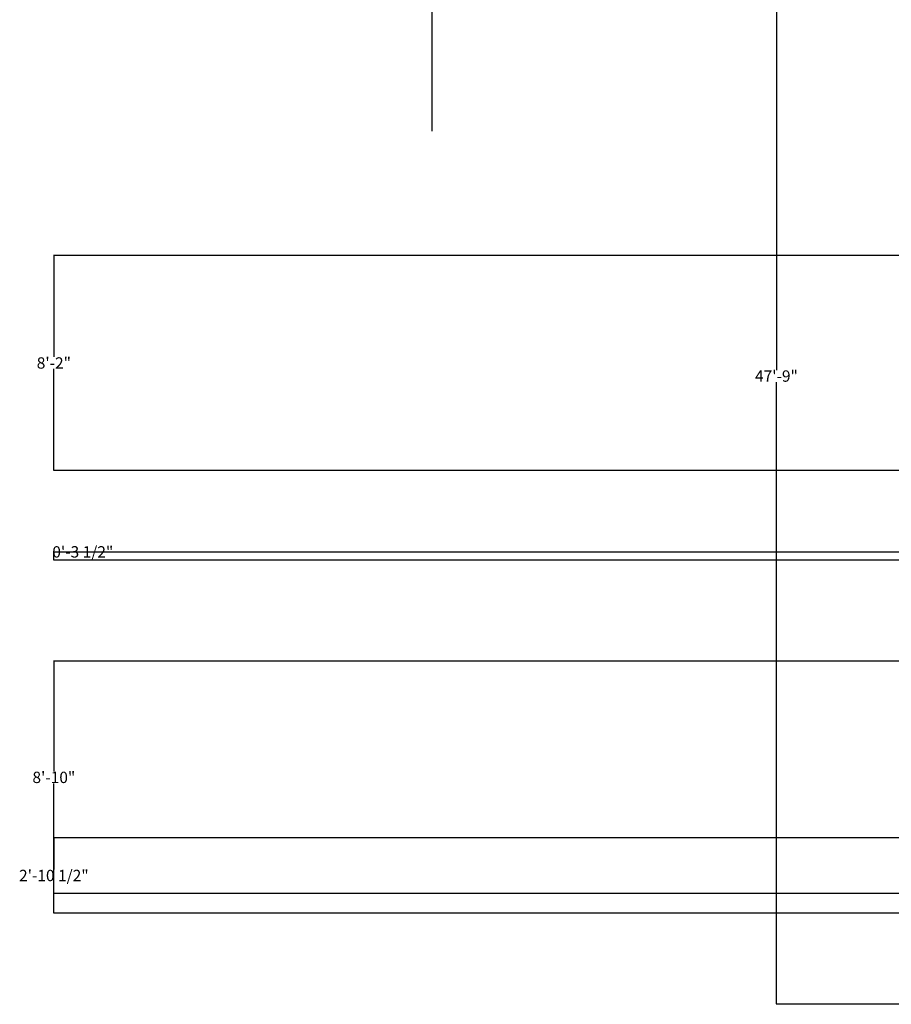
# Model space of a CAD drawing. Units: inches. Extents: x -157 to 1464, y -361 to 1077.
# Tile 1 of 9: x -157 to 241, y 70 to 519. Entities that reach past the tile are written whole.
import ezdxf

# ---------------------------------------------------------------- set-up
doc = ezdxf.new("R2010")
doc.units = ezdxf.units.IN
doc.header["$MEASUREMENT"] = 0
for name, color, linetype, lineweight in [('A-ANNO-DIMS', 2, 'Continuous', 18), ('C-ANNO-DIMS', 2, 'Continuous', 18), ('C-ROAD', 7, 'Continuous', 25)]:
    doc.layers.add(name, color=color, linetype=linetype, lineweight=lineweight)
doc.styles.get("Standard").update_dxf_attribs({"font": 'arial.ttf'})
doc.dimstyles.new('Annotative', dxfattribs={"dimscale": 0, "dimtxt": 5.18, "dimasz": 0.18, "dimexe": 0.18, "dimexo": 0.0625, "dimgap": 0.09, "dimtad": 0, "dimtih": 1, "dimtoh": 1, "dimdec": 0, "dimzin": 0, "dimdsep": 46, "dimlunit": 3, "dimtxsty": 'Standard', "dimcen": 0.09, "dimadec": 0, "dimazin": 0, "dimtfac": 1, "dimtdec": 0, "dimtofl": 0, "dimtmove": 0, "dimatfit": 3, "dimfxl": 1, "dimtolj": 1, "dimtzin": 0, "dimarcsym": 0})

# ---------------------------------------------------------------- blocks, each defined once
blk = doc.blocks.new('*D13')
at = {"layer": 'C-ANNO-DIMS', "color": 0, "lineweight": -2, "transparency": 16777216}
for p, q in [((257.27, 643.42), (188.08, 643.42)), ((188.26, 643.24), (188.26, 359.63)), ((188.26, 70.55), (188.26, 354.16)), ((257.27, 70.37), (188.08, 70.37))]:
    blk.add_line(p, q, dxfattribs=at)
at = {"layer": 'C-ANNO-DIMS', "color": 0, "transparency": 16777216}
for points in [[(188.23, 643.24), (188.29, 643.24), (188.26, 643.42)], [(188.23, 70.55), (188.29, 70.55), (188.26, 70.37)]]:
    blk.add_solid(points, dxfattribs=at)
at = {"layer": 'Defpoints', "color": 0, "transparency": 16777216}
for p in [(257.33, 643.42), (188.26, 70.37), (257.33, 70.37)]:
    blk.add_point(p, dxfattribs=at)
at = {"layer": 'C-ANNO-DIMS', "color": 0, "transparency": 16777216, "insert": (188.26, 356.89), "char_height": 5.18, "attachment_point": 5}
blk.add_mtext('\\A1;47\'-9"', dxfattribs=at)
blk = doc.blocks.new('*D71')
at = {"layer": 'A-ANNO-DIMS', "color": 0, "lineweight": -2, "transparency": 16777216}
for p, q in [((298.9, 146.36), (-141.39, 146.36)), ((-141.21, 146.18), (-141.21, 131.88)), ((-141.21, 112.04), (-141.21, 126.34)), ((298.9, 111.86), (-141.39, 111.86))]:
    blk.add_line(p, q, dxfattribs=at)
at = {"layer": 'A-ANNO-DIMS', "color": 0, "transparency": 16777216}
for points in [[(-141.24, 146.18), (-141.18, 146.18), (-141.21, 146.36)], [(-141.24, 112.04), (-141.18, 112.04), (-141.21, 111.86)]]:
    blk.add_solid(points, dxfattribs=at)
at = {"layer": 'Defpoints', "color": 0, "transparency": 16777216}
for p in [(-141.21, 146.36), (298.97, 146.36), (298.97, 111.86)]:
    blk.add_point(p, dxfattribs=at)
at = {"layer": 'A-ANNO-DIMS', "color": 0, "transparency": 16777216, "insert": (-141.21, 129.11), "char_height": 5.18, "attachment_point": 5}
blk.add_mtext('\\A1;2\'-10 1/2"', dxfattribs=at)
blk = doc.blocks.new('*D72')
at = {"layer": 'A-ANNO-DIMS', "color": 0, "lineweight": -2, "transparency": 16777216}
for p, q in [((298.9, 276.53), (-141.39, 276.53)), ((-141.21, 276.53), (-141.21, 276.71)), ((-141.21, 276.71), (-141.03, 276.71)), ((-141.21, 273.04), (-141.21, 276.35)), ((307.9, 272.86), (-141.39, 272.86))]:
    blk.add_line(p, q, dxfattribs=at)
at = {"layer": 'A-ANNO-DIMS', "color": 0, "transparency": 16777216}
for points in [[(-141.24, 276.35), (-141.18, 276.35), (-141.21, 276.53)], [(-141.24, 273.04), (-141.18, 273.04), (-141.21, 272.86)]]:
    blk.add_solid(points, dxfattribs=at)
at = {"layer": 'Defpoints', "color": 0, "transparency": 16777216}
for p in [(-141.21, 276.53), (298.97, 276.53), (307.97, 272.86)]:
    blk.add_point(p, dxfattribs=at)
at = {"layer": 'A-ANNO-DIMS', "color": 0, "transparency": 16777216, "insert": (-128.02, 276.71), "char_height": 5.18, "attachment_point": 5}
blk.add_mtext('\\A1;0\'-3 1/2"', dxfattribs=at)
blk = doc.blocks.new('*D77')
at = {"layer": 'A-ANNO-DIMS', "color": 0, "lineweight": -2, "transparency": 16777216}
for p, q in [((427.9, 411.86), (-141.39, 411.86)), ((-141.21, 411.68), (-141.21, 365.6)), ((-141.21, 314.04), (-141.21, 360.13)), ((427.9, 313.86), (-141.39, 313.86))]:
    blk.add_line(p, q, dxfattribs=at)
at = {"layer": 'A-ANNO-DIMS', "color": 0, "transparency": 16777216}
for points in [[(-141.24, 411.68), (-141.18, 411.68), (-141.21, 411.86)], [(-141.24, 314.04), (-141.18, 314.04), (-141.21, 313.86)]]:
    blk.add_solid(points, dxfattribs=at)
at = {"layer": 'Defpoints', "color": 0, "transparency": 16777216}
for p in [(-141.21, 411.86), (427.97, 411.86), (427.97, 313.86)]:
    blk.add_point(p, dxfattribs=at)
at = {"layer": 'A-ANNO-DIMS', "color": 0, "transparency": 16777216, "insert": (-141.21, 362.86), "char_height": 5.18, "attachment_point": 5}
blk.add_mtext('\\A1;8\'-2"', dxfattribs=at)
blk = doc.blocks.new('*D78')
at = {"layer": 'A-ANNO-DIMS', "color": 0, "lineweight": -2, "transparency": 16777216}
for p, q in [((427.9, 226.86), (-141.39, 226.86)), ((-141.21, 226.68), (-141.21, 176.6)), ((-141.21, 121.04), (-141.21, 171.13)), ((427.9, 120.86), (-141.39, 120.86))]:
    blk.add_line(p, q, dxfattribs=at)
at = {"layer": 'A-ANNO-DIMS', "color": 0, "transparency": 16777216}
for points in [[(-141.24, 226.68), (-141.18, 226.68), (-141.21, 226.86)], [(-141.24, 121.04), (-141.18, 121.04), (-141.21, 120.86)]]:
    blk.add_solid(points, dxfattribs=at)
at = {"layer": 'Defpoints', "color": 0, "transparency": 16777216}
for p in [(427.97, 226.86), (-141.21, 120.86), (427.97, 120.86)]:
    blk.add_point(p, dxfattribs=at)
at = {"layer": 'A-ANNO-DIMS', "color": 0, "transparency": 16777216, "insert": (-141.21, 173.86), "char_height": 5.18, "attachment_point": 5}
blk.add_mtext('\\A1;8\'-10"', dxfattribs=at)

msp = doc.modelspace()

# ---------------------------------------------------------------- linework, layer by layer
at = {"layer": 'C-ROAD'}
msp.add_line((31.23, 468.62), (31.23, 704.11), dxfattribs=at)

# ---------------------------------------------------------------- dimensions: what is measured, and where the dimension line sits
at = {"layer": 'A-ANNO-DIMS'}
for base, p1, p2, picture, middle in [((-141.21, 411.86), (427.97, 313.86), (427.97, 411.86), '*D77', (-141.21, 362.86)), ((-141.21, 276.53), (307.97, 272.86), (298.97, 276.53), '*D72', (-128.02, 276.71)), ((-141.21, 120.86), (427.97, 226.86), (427.97, 120.86), '*D78', (-141.21, 173.86)), ((-141.21, 146.36), (298.97, 111.86), (298.97, 146.36), '*D71', (-141.21, 129.11))]:
    dim = msp.add_linear_dim(base=base, p1=p1, p2=p2, angle=90, dimstyle='Annotative', override={"dimscale": 1, "dimdec": 1, "dimzin": 1, "dimlunit": 4, "dimfrac": 2}, dxfattribs=at)
    dim.commit()
    dim.dimension.update_dxf_attribs({"geometry": picture, "text_midpoint": middle})
at = {"layer": 'C-ANNO-DIMS'}
dim = msp.add_linear_dim(base=(188.26, 70.37), p1=(257.33, 643.42), p2=(257.33, 70.37), angle=90, dimstyle='Annotative', override={"dimclrd": 0, "dimclre": 0, "dimclrt": 0}, dxfattribs=at)
dim.commit()
dim.dimension.update_dxf_attribs({"geometry": '*D13', "text_midpoint": (188.26, 356.89)})

doc.saveas('drawing.dxf')
